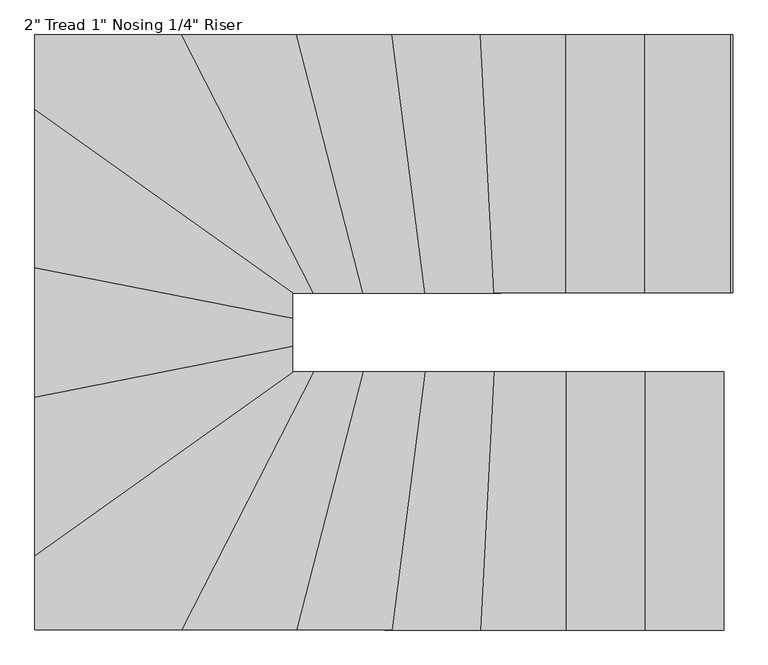
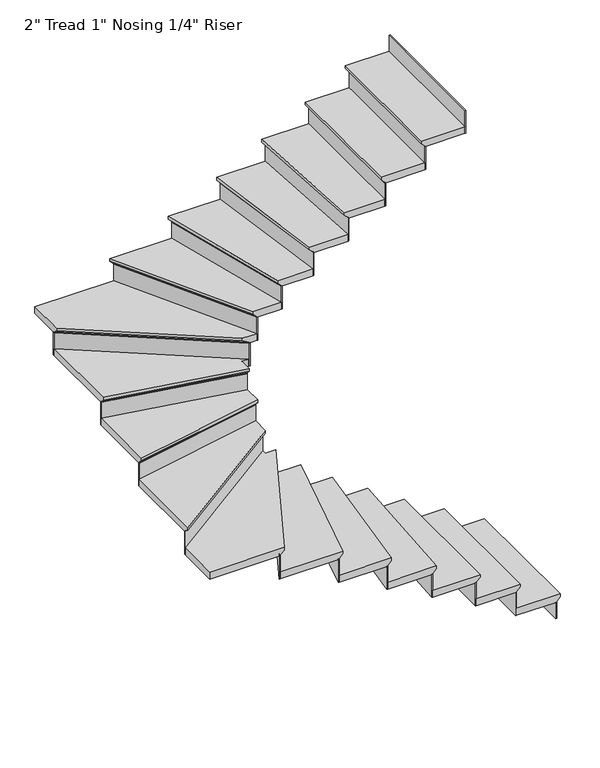
"""IFC4 building model written with IfcOpenShell, lengths in millimetres: stair flight geometry."""

from ifc_helpers import new_model, si_unit, origin, place, context, project, spatial, faceted_brep, source, transform, mapped, element, save


def stair_flight_428a4bf9(model_context):
    return source(origin(), model_context, "Body", "Brep", [
        faceted_brep([(-1761.7449167, -345.7070853, 6551.0833333), (-1761.7449167, -345.7070853, 6570.1333333), (-1761.7449167, -1260.1070853, 6570.1333333), (-1761.7449167, -1260.1070853, 6551.0833333), (-1787.1449167, -345.7070853, 6525.6833333), (-1787.1449167, -1260.1070853, 6525.6833333), (-2066.5449167, -345.7070853, 6570.1333333), (-2066.5449167, -1260.1070853, 6570.1333333), (-1787.1449167, -1260.1070853, 6519.3333333), (-2066.5449167, -1260.1070853, 6519.3333333), (-2066.5449167, -345.7070853, 6519.3333333), (-1787.1449167, -345.7070853, 6519.3333333)], [[[0, 1, 2, 3]], [[4, 0, 3, 5]], [[2, 1, 6, 7]], [[8, 9, 10, 11]], [[2, 7, 9, 8, 5, 3]], [[8, 11, 4, 5]], [[6, 1, 0, 4, 11, 10]], [[7, 6, 10, 9]]]),
        faceted_brep([(-1787.1449167, -345.7070853, 6519.3333333), (-1787.1449167, -345.7070853, 6400.8), (-1793.4949167, -345.7070853, 6400.8), (-1793.4949167, -345.7070853, 6519.3333333), (-1787.1449167, -1260.1070853, 6519.3333333), (-1793.4949167, -1260.1070853, 6519.3333333), (-1793.4949167, -1260.1070853, 6400.8), (-1787.1449167, -1260.1070853, 6400.8)], [[[0, 1, 2, 3]], [[4, 5, 6, 7]], [[1, 0, 4, 7]], [[2, 1, 7, 6]], [[3, 2, 6, 5]], [[0, 3, 5, 4]]]),
        faceted_brep([(-2066.5449167, -345.7070853, 6688.6666667), (-2066.5449167, -345.7070853, 6519.3333333), (-2072.8949167, -345.7070853, 6519.3333333), (-2072.8949167, -345.7070853, 6688.6666667), (-2066.5449167, -1260.1070853, 6688.6666667), (-2072.8949167, -1260.1070853, 6688.6666667), (-2072.8949167, -1260.1070853, 6519.3333333), (-2066.5449167, -1260.1070853, 6519.3333333)], [[[0, 1, 2, 3]], [[4, 5, 6, 7]], [[1, 0, 4, 7]], [[2, 1, 7, 6]], [[3, 2, 6, 5]], [[0, 3, 5, 4]]]),
        faceted_brep([(-2041.1449167, -1260.1070853, 6739.4666667), (-2041.1449167, -345.7070853, 6739.4666667), (-2345.9449167, -345.7070853, 6739.4666667), (-2345.9449167, -1260.1070853, 6739.4666667), (-2066.5449167, -1260.1070853, 6688.6666667), (-2345.9449167, -1260.1070853, 6688.6666667), (-2345.9449167, -345.7070853, 6688.6666667), (-2066.5449167, -345.7070853, 6688.6666667), (-2066.5449167, -1260.1070853, 6695.0166667), (-2041.1449167, -1260.1070853, 6720.4166667), (-2066.5449167, -345.7070853, 6695.0166667), (-2041.1449167, -345.7070853, 6720.4166667)], [[[0, 1, 2, 3]], [[4, 5, 6, 7]], [[0, 3, 5, 4, 8, 9]], [[4, 7, 10, 8]], [[2, 1, 11, 10, 7, 6]], [[3, 2, 6, 5]], [[11, 1, 0, 9]], [[10, 11, 9, 8]]]),
        faceted_brep([(-2345.9449167, -345.7070853, 6858.0), (-2345.9449167, -345.7070853, 6688.6666667), (-2352.2949167, -345.7070853, 6688.6666667), (-2352.2949167, -345.7070853, 6858.0), (-2345.9449167, -1260.1070853, 6858.0), (-2352.2949167, -1260.1070853, 6858.0), (-2352.2949167, -1260.1070853, 6688.6666667), (-2345.9449167, -1260.1070853, 6688.6666667)], [[[0, 1, 2, 3]], [[4, 5, 6, 7]], [[1, 0, 4, 7]], [[2, 1, 7, 6]], [[3, 2, 6, 5]], [[0, 3, 5, 4]]]),
        faceted_brep([(-2320.5449167, -1260.1070853, 6908.8), (-2320.5449167, -345.7070853, 6908.8), (-2601.6120781, -345.7070853, 6908.8), (-2649.1463485, -1260.1070853, 6908.8), (-2345.9449167, -1260.1070853, 6858.0), (-2649.1463485, -1260.1070853, 6858.0), (-2601.6120781, -345.7070853, 6858.0), (-2345.9449167, -345.7070853, 6858.0), (-2345.9449167, -1260.1070853, 6864.35), (-2320.5449167, -1260.1070853, 6889.75), (-2345.9449167, -345.7070853, 6864.35), (-2320.5449167, -345.7070853, 6889.75)], [[[0, 1, 2, 3]], [[4, 5, 6, 7]], [[0, 3, 5, 4, 8, 9]], [[4, 7, 10, 8]], [[2, 1, 11, 10, 7, 6]], [[3, 2, 6, 5]], [[11, 1, 0, 9]], [[10, 11, 9, 8]]]),
        faceted_brep([(-2601.6120781, -345.7070853, 7027.3333333), (-2601.6120781, -345.7070853, 6858.0), (-2607.9706523, -345.7070853, 6858.0), (-2607.9706523, -345.7070853, 7027.3333333), (-2649.1463485, -1260.1070853, 7027.3333333), (-2655.5049227, -1260.1070853, 7027.3333333), (-2655.5049227, -1260.1070853, 6858.0), (-2649.1463485, -1260.1070853, 6858.0)], [[[0, 1, 2, 3]], [[4, 5, 6, 7]], [[1, 0, 4, 7]], [[2, 1, 7, 6]], [[3, 2, 6, 5]], [[0, 3, 5, 4]]]),
        faceted_brep([(-2623.7120519, -1260.1070853, 7078.1333333), (-2576.1777815, -345.7070853, 7078.1333333), (-2845.778778, -345.7070853, 7078.1333333), (-2964.1348296, -1260.1070853, 7078.1333333), (-2649.1463485, -1260.1070853, 7027.3333333), (-2964.1348296, -1260.1070853, 7027.3333333), (-2845.778778, -345.7070853, 7027.3333333), (-2601.6120781, -345.7070853, 7027.3333333), (-2649.1463485, -1260.1070853, 7033.6833333), (-2623.7120519, -1260.1070853, 7059.0833333), (-2601.6120781, -345.7070853, 7033.6833333), (-2576.1777815, -345.7070853, 7059.0833333)], [[[0, 1, 2, 3]], [[4, 5, 6, 7]], [[0, 3, 5, 4, 8, 9]], [[4, 7, 10, 8]], [[2, 1, 11, 10, 7, 6]], [[3, 2, 6, 5]], [[11, 1, 0, 9]], [[10, 11, 9, 8]]]),
        faceted_brep([(-2845.778778, -345.7070853, 7196.6666667), (-2845.778778, -345.7070853, 7027.3333333), (-2852.1817497, -345.7070853, 7027.3333333), (-2852.1817497, -345.7070853, 7196.6666667), (-2964.1348296, -1260.1070853, 7196.6666667), (-2970.5378014, -1260.1070853, 7196.6666667), (-2970.5378014, -1260.1070853, 7027.3333333), (-2964.1348296, -1260.1070853, 7027.3333333)], [[[0, 1, 2, 3]], [[4, 5, 6, 7]], [[1, 0, 4, 7]], [[2, 1, 7, 6]], [[3, 2, 6, 5]], [[0, 3, 5, 4]]]),
        faceted_brep([(-2938.5229425, -1260.1070853, 7247.4666667), (-2820.1668908, -345.7070853, 7247.4666667), (-3067.4060004, -345.7070853, 7247.4666667), (-3302.5364478, -1260.1070853, 7247.4666667), (-2964.1348296, -1260.1070853, 7196.6666667), (-3302.5364478, -1260.1070853, 7196.6666667), (-3067.4060004, -345.7070853, 7196.6666667), (-2845.778778, -345.7070853, 7196.6666667), (-2964.1348296, -1260.1070853, 7203.0166667), (-2938.5229425, -1260.1070853, 7228.4166667), (-2845.778778, -345.7070853, 7203.0166667), (-2820.1668908, -345.7070853, 7228.4166667)], [[[0, 1, 2, 3]], [[4, 5, 6, 7]], [[0, 3, 5, 4, 8, 9]], [[4, 7, 10, 8]], [[2, 1, 11, 10, 7, 6]], [[3, 2, 6, 5]], [[11, 1, 0, 9]], [[10, 11, 9, 8]]]),
        faceted_brep([(-3067.4060004, -345.7070853, 7366.0), (-3067.4060004, -345.7070853, 7196.6666667), (-3073.9625773, -345.7070853, 7196.6666667), (-3073.9625773, -345.7070853, 7366.0), (-3302.5364478, -1260.1070853, 7366.0), (-3309.0930247, -1260.1070853, 7366.0), (-3309.0930247, -1260.1070853, 7196.6666667), (-3302.5364478, -1260.1070853, 7196.6666667)], [[[0, 1, 2, 3]], [[4, 5, 6, 7]], [[1, 0, 4, 7]], [[2, 1, 7, 6]], [[3, 2, 6, 5]], [[0, 3, 5, 4]]]),
        faceted_brep([(-3276.3101404, -1260.1070853, 7416.8), (-3041.179693, -345.7070853, 7416.8), (-3243.7526365, -345.7070853, 7416.8), (-3712.5772578, -1260.1070853, 7416.8), (-3302.5364478, -1260.1070853, 7366.0), (-3712.5772578, -1260.1070853, 7366.0), (-3243.7526365, -345.7070853, 7366.0), (-3067.4060004, -345.7070853, 7366.0), (-3302.5364478, -1260.1070853, 7372.35), (-3276.3101404, -1260.1070853, 7397.75), (-3067.4060004, -345.7070853, 7372.35), (-3041.179693, -345.7070853, 7397.75)], [[[0, 1, 2, 3]], [[4, 5, 6, 7]], [[0, 3, 5, 4, 8, 9]], [[4, 7, 10, 8]], [[2, 1, 11, 10, 7, 6]], [[3, 2, 6, 5]], [[11, 1, 0, 9]], [[10, 11, 9, 8]]]),
        faceted_brep([(-3243.7526365, -345.7070853, 7535.3333333), (-3243.7526365, -345.7070853, 7366.0), (-3250.8886197, -345.7070853, 7366.0), (-3250.8886197, -345.7070853, 7535.3333333), (-3712.5772578, -1260.1070853, 7535.3333333), (-3719.713241, -1260.1070853, 7535.3333333), (-3719.713241, -1260.1070853, 7366.0), (-3712.5772578, -1260.1070853, 7366.0)], [[[0, 1, 2, 3]], [[4, 5, 6, 7]], [[1, 0, 4, 7]], [[2, 1, 7, 6]], [[3, 2, 6, 5]], [[0, 3, 5, 4]]]),
        faceted_brep([(-4203.8766085, -966.4259516, 7586.1333333), (-4203.8766085, -1260.1070853, 7586.1333333), (-3684.0333253, -1260.1070853, 7586.1333333), (-3215.208704, -345.7070853, 7586.1333333), (-3289.4766085, -345.7070853, 7586.1333333), (-3289.4766085, -316.1520025, 7586.1333333), (-4203.8766085, -1260.1070853, 7535.3333333), (-4203.8766085, -966.4259516, 7535.3333333), (-3289.4766085, -316.1520025, 7535.3333333), (-3289.4766085, -345.7070853, 7535.3333333), (-3243.7526365, -345.7070853, 7535.3333333), (-3712.5772578, -1260.1070853, 7535.3333333), (-3712.5772578, -1260.1070853, 7541.6833333), (-3684.0333253, -1260.1070853, 7567.0833333), (-3243.7526365, -345.7070853, 7541.6833333), (-3215.208704, -345.7070853, 7567.0833333)], [[[0, 1, 2, 3, 4, 5]], [[6, 7, 8, 9, 10, 11]], [[1, 0, 7, 6]], [[2, 1, 6, 11, 12, 13]], [[11, 10, 14, 12]], [[4, 3, 15, 14, 10, 9]], [[5, 4, 9, 8]], [[0, 5, 8, 7]], [[15, 3, 2, 13]], [[14, 15, 13, 12]]]),
        faceted_brep([(-3289.4766085, -316.1520025, 7704.6666667), (-3289.4766085, -316.1520025, 7535.3333333), (-3289.4766085, -308.3600277, 7535.3333333), (-3289.4766085, -308.3600277, 7704.6666667), (-4203.8766085, -966.4259516, 7704.6666667), (-4203.8766085, -958.6339768, 7704.6666667), (-4203.8766085, -958.6339768, 7535.3333333), (-4203.8766085, -966.4259516, 7535.3333333)], [[[0, 1, 2, 3]], [[4, 5, 6, 7]], [[1, 0, 4, 7]], [[2, 1, 7, 6]], [[3, 2, 6, 5]], [[0, 3, 5, 4]]]),
        faceted_brep([(-4203.8766085, -997.5938508, 7755.4666667), (-3289.4766085, -347.3199017, 7755.4666667), (-3289.4766085, -229.6979154, 7755.4666667), (-4203.8766085, -409.9387717, 7755.4666667), (-4203.8766085, -966.4259516, 7704.6666667), (-4203.8766085, -409.9387717, 7704.6666667), (-3289.4766085, -229.6979154, 7704.6666667), (-3289.4766085, -316.1520025, 7704.6666667), (-4203.8766085, -966.4259516, 7711.0166667), (-4203.8766085, -997.5938508, 7736.4166667), (-3289.4766085, -316.1520025, 7711.0166667), (-3289.4766085, -347.3199017, 7736.4166667)], [[[0, 1, 2, 3]], [[4, 5, 6, 7]], [[0, 3, 5, 4, 8, 9]], [[4, 7, 10, 8]], [[2, 1, 11, 10, 7, 6]], [[3, 2, 6, 5]], [[11, 1, 0, 9]], [[10, 11, 9, 8]]]),
        faceted_brep([(-3289.4766085, -229.6979154, 7874.0), (-3289.4766085, -229.6979154, 7704.6666667), (-3289.4766085, -223.22573, 7704.6666667), (-3289.4766085, -223.22573, 7874.0), (-4203.8766085, -409.9387717, 7874.0), (-4203.8766085, -403.4665863, 7874.0), (-4203.8766085, -403.4665863, 7704.6666667), (-4203.8766085, -409.9387717, 7704.6666667)], [[[0, 1, 2, 3]], [[4, 5, 6, 7]], [[1, 0, 4, 7]], [[2, 1, 7, 6]], [[3, 2, 6, 5]], [[0, 3, 5, 4]]]),
        faceted_brep([(-4203.8766085, -435.8275135, 7924.8), (-3289.4766085, -255.5866572, 7924.8), (-3289.4766085, -130.5387717, 7924.8), (-4203.8766085, 49.7020846, 7924.8), (-4203.8766085, -409.9387717, 7874.0), (-4203.8766085, 49.7020846, 7874.0), (-3289.4766085, -130.5387717, 7874.0), (-3289.4766085, -229.6979154, 7874.0), (-4203.8766085, -409.9387717, 7880.35), (-4203.8766085, -435.8275135, 7905.75), (-3289.4766085, -229.6979154, 7880.35), (-3289.4766085, -255.5866572, 7905.75)], [[[0, 1, 2, 3]], [[4, 5, 6, 7]], [[0, 3, 5, 4, 8, 9]], [[4, 7, 10, 8]], [[2, 1, 11, 10, 7, 6]], [[3, 2, 6, 5]], [[11, 1, 0, 9]], [[10, 11, 9, 8]]]),
        faceted_brep([(-3289.4766085, -130.5387717, 8043.3333333), (-3289.4766085, -130.5387717, 7874.0), (-3289.4766085, -124.0665863, 7874.0), (-3289.4766085, -124.0665863, 8043.3333333), (-4203.8766085, 49.7020846, 8043.3333333), (-4203.8766085, 56.17427, 8043.3333333), (-4203.8766085, 56.17427, 7874.0), (-4203.8766085, 49.7020846, 7874.0)], [[[0, 1, 2, 3]], [[4, 5, 6, 7]], [[1, 0, 4, 7]], [[2, 1, 7, 6]], [[3, 2, 6, 5]], [[0, 3, 5, 4]]]),
        faceted_brep([(-4203.8766085, 23.8133428, 8094.1333333), (-3289.4766085, -156.4275135, 8094.1333333), (-3289.4766085, -66.3070853, 8094.1333333), (-3243.381134, -66.3070853, 8094.1333333), (-4203.8766085, 616.7475793, 8094.1333333), (-4203.8766085, 49.7020846, 8043.3333333), (-4203.8766085, 616.7475793, 8043.3333333), (-3243.381134, -66.3070853, 8043.3333333), (-3289.4766085, -66.3070853, 8043.3333333), (-3289.4766085, -130.5387717, 8043.3333333), (-4203.8766085, 49.7020846, 8049.6833333), (-4203.8766085, 23.8133428, 8075.0833333), (-3289.4766085, -130.5387717, 8049.6833333), (-3289.4766085, -156.4275135, 8075.0833333)], [[[0, 1, 2, 3, 4]], [[5, 6, 7, 8, 9]], [[0, 4, 6, 5, 10, 11]], [[5, 9, 12, 10]], [[2, 1, 13, 12, 9, 8]], [[3, 2, 8, 7]], [[4, 3, 7, 6]], [[13, 1, 0, 11]], [[12, 13, 11, 10]]]),
        faceted_brep([(-3243.381134, -66.3070853, 8212.6666667), (-3243.381134, -66.3070853, 8043.3333333), (-3232.4242415, -66.3070853, 8043.3333333), (-3232.4242415, -66.3070853, 8212.6666667), (-4203.8766085, 616.7475793, 8212.6666667), (-4203.8766085, 624.5395541, 8212.6666667), (-4203.8766085, 624.5395541, 8043.3333333), (-4203.8766085, 616.7475793, 8043.3333333)], [[[0, 1, 2, 3]], [[4, 5, 6, 7]], [[1, 0, 4, 7]], [[2, 1, 7, 6]], [[3, 2, 6, 5]], [[0, 3, 5, 4]]]),
        faceted_brep([(-3655.4893928, 848.0929147, 8263.4666667), (-4203.8766085, 848.0929147, 8263.4666667), (-4203.8766085, 585.5796802, 8263.4666667), (-3287.208704, -66.3070853, 8263.4666667), (-3186.6647715, -66.3070853, 8263.4666667), (-4203.8766085, 848.0929147, 8212.6666667), (-3655.4893928, 848.0929147, 8212.6666667), (-3186.6647715, -66.3070853, 8212.6666667), (-3243.381134, -66.3070853, 8212.6666667), (-4203.8766085, 616.7475793, 8212.6666667), (-4203.8766085, 616.7475793, 8219.0166667), (-4203.8766085, 585.5796802, 8244.4166667), (-3243.381134, -66.3070853, 8219.0166667), (-3287.208704, -66.3070853, 8244.4166667)], [[[0, 1, 2, 3, 4]], [[5, 6, 7, 8, 9]], [[1, 0, 6, 5]], [[2, 1, 5, 9, 10, 11]], [[9, 8, 12, 10]], [[4, 3, 13, 12, 8, 7]], [[0, 4, 7, 6]], [[13, 3, 2, 11]], [[12, 13, 11, 10]]]),
        faceted_brep([(-3186.6647715, -66.3070853, 8382.0), (-3186.6647715, -66.3070853, 8212.6666667), (-3179.5287883, -66.3070853, 8212.6666667), (-3179.5287883, -66.3070853, 8382.0), (-3655.4893928, 848.0929147, 8382.0), (-3648.3534096, 848.0929147, 8382.0), (-3648.3534096, 848.0929147, 8212.6666667), (-3655.4893928, 848.0929147, 8212.6666667)], [[[0, 1, 2, 3]], [[4, 5, 6, 7]], [[1, 0, 4, 7]], [[2, 1, 7, 6]], [[3, 2, 6, 5]], [[0, 3, 5, 4]]]),
        faceted_brep([(-3684.0333253, 848.0929147, 8432.8), (-3215.208704, -66.3070853, 8432.8), (-3014.9533855, -66.3070853, 8432.8), (-3250.0838329, 848.0929147, 8432.8), (-3655.4893928, 848.0929147, 8382.0), (-3250.0838329, 848.0929147, 8382.0), (-3014.9533855, -66.3070853, 8382.0), (-3186.6647715, -66.3070853, 8382.0), (-3655.4893928, 848.0929147, 8388.35), (-3684.0333253, 848.0929147, 8413.75), (-3186.6647715, -66.3070853, 8388.35), (-3215.208704, -66.3070853, 8413.75)], [[[0, 1, 2, 3]], [[4, 5, 6, 7]], [[0, 3, 5, 4, 8, 9]], [[4, 7, 10, 8]], [[2, 1, 11, 10, 7, 6]], [[3, 2, 6, 5]], [[11, 1, 0, 9]], [[10, 11, 9, 8]]]),
        faceted_brep([(-3014.9533855, -66.3070853, 8551.3333333), (-3014.9533855, -66.3070853, 8382.0), (-3008.3968086, -66.3070853, 8382.0), (-3008.3968086, -66.3070853, 8551.3333333), (-3250.0838329, 848.0929147, 8551.3333333), (-3243.5272561, 848.0929147, 8551.3333333), (-3243.5272561, 848.0929147, 8382.0), (-3250.0838329, 848.0929147, 8382.0)], [[[0, 1, 2, 3]], [[4, 5, 6, 7]], [[1, 0, 4, 7]], [[2, 1, 7, 6]], [[3, 2, 6, 5]], [[0, 3, 5, 4]]]),
        faceted_brep([(-3276.3101404, 848.0929147, 8602.1333333), (-3041.179693, -66.3070853, 8602.1333333), (-2794.5550037, -66.3070853, 8602.1333333), (-2912.9110554, 848.0929147, 8602.1333333), (-3250.0838329, 848.0929147, 8551.3333333), (-2912.9110554, 848.0929147, 8551.3333333), (-2794.5550037, -66.3070853, 8551.3333333), (-3014.9533855, -66.3070853, 8551.3333333), (-3250.0838329, 848.0929147, 8557.6833333), (-3276.3101404, 848.0929147, 8583.0833333), (-3014.9533855, -66.3070853, 8557.6833333), (-3041.179693, -66.3070853, 8583.0833333)], [[[0, 1, 2, 3]], [[4, 5, 6, 7]], [[0, 3, 5, 4, 8, 9]], [[4, 7, 10, 8]], [[2, 1, 11, 10, 7, 6]], [[3, 2, 6, 5]], [[11, 1, 0, 9]], [[10, 11, 9, 8]]]),
        faceted_brep([(-2794.5550037, -66.3070853, 8720.6666667), (-2794.5550037, -66.3070853, 8551.3333333), (-2788.152032, -66.3070853, 8551.3333333), (-2788.152032, -66.3070853, 8720.6666667), (-2912.9110554, 848.0929147, 8720.6666667), (-2906.5080836, 848.0929147, 8720.6666667), (-2906.5080836, 848.0929147, 8551.3333333), (-2912.9110554, 848.0929147, 8551.3333333)], [[[0, 1, 2, 3]], [[4, 5, 6, 7]], [[1, 0, 4, 7]], [[2, 1, 7, 6]], [[3, 2, 6, 5]], [[0, 3, 5, 4]]]),
        faceted_brep([(-2938.5229425, 848.0929147, 8771.4666667), (-2820.1668908, -66.3070853, 8771.4666667), (-2550.7434848, -66.3070853, 8771.4666667), (-2598.2777552, 848.0929147, 8771.4666667), (-2912.9110554, 848.0929147, 8720.6666667), (-2598.2777552, 848.0929147, 8720.6666667), (-2550.7434848, -66.3070853, 8720.6666667), (-2794.5550037, -66.3070853, 8720.6666667), (-2912.9110554, 848.0929147, 8727.0166667), (-2938.5229425, 848.0929147, 8752.4166667), (-2794.5550037, -66.3070853, 8727.0166667), (-2820.1668908, -66.3070853, 8752.4166667)], [[[0, 1, 2, 3]], [[4, 5, 6, 7]], [[0, 3, 5, 4, 8, 9]], [[4, 7, 10, 8]], [[2, 1, 11, 10, 7, 6]], [[3, 2, 6, 5]], [[11, 1, 0, 9]], [[10, 11, 9, 8]]]),
        faceted_brep([(-2550.7434848, -66.3070853, 8890.0), (-2550.7434848, -66.3070853, 8720.6666667), (-2544.3849106, -66.3070853, 8720.6666667), (-2544.3849106, -66.3070853, 8890.0), (-2598.2777552, 848.0929147, 8890.0), (-2591.9191811, 848.0929147, 8890.0), (-2591.9191811, 848.0929147, 8720.6666667), (-2598.2777552, 848.0929147, 8720.6666667)], [[[0, 1, 2, 3]], [[4, 5, 6, 7]], [[1, 0, 4, 7]], [[2, 1, 7, 6]], [[3, 2, 6, 5]], [[0, 3, 5, 4]]]),
        faceted_brep([(-2623.7120519, 848.0929147, 8940.8), (-2576.1777815, -66.3070853, 8940.8), (-2295.1449167, -66.3070853, 8940.8), (-2295.1449167, 848.0929147, 8940.8), (-2598.2777552, 848.0929147, 8890.0), (-2295.1449167, 848.0929147, 8890.0), (-2295.1449167, -66.3070853, 8890.0), (-2550.7434848, -66.3070853, 8890.0), (-2598.2777552, 848.0929147, 8896.35), (-2623.7120519, 848.0929147, 8921.75), (-2550.7434848, -66.3070853, 8896.35), (-2576.1777815, -66.3070853, 8921.75)], [[[0, 1, 2, 3]], [[4, 5, 6, 7]], [[0, 3, 5, 4, 8, 9]], [[4, 7, 10, 8]], [[2, 1, 11, 10, 7, 6]], [[3, 2, 6, 5]], [[11, 1, 0, 9]], [[10, 11, 9, 8]]]),
        faceted_brep([(-2295.1449167, -66.3070853, 9059.3333333), (-2295.1449167, -66.3070853, 8890.0), (-2288.7949167, -66.3070853, 8890.0), (-2288.7949167, -66.3070853, 9059.3333333), (-2295.1449167, 848.0929147, 9059.3333333), (-2288.7949167, 848.0929147, 9059.3333333), (-2288.7949167, 848.0929147, 8890.0), (-2295.1449167, 848.0929147, 8890.0)], [[[0, 1, 2, 3]], [[4, 5, 6, 7]], [[1, 0, 4, 7]], [[2, 1, 7, 6]], [[3, 2, 6, 5]], [[0, 3, 5, 4]]]),
        faceted_brep([(-2320.5449167, 848.0929147, 9110.1333333), (-2320.5449167, -66.3070853, 9110.1333333), (-2015.7449167, -66.3070853, 9110.1333333), (-2015.7449167, 848.0929147, 9110.1333333), (-2295.1449167, 848.0929147, 9059.3333333), (-2015.7449167, 848.0929147, 9059.3333333), (-2015.7449167, -66.3070853, 9059.3333333), (-2295.1449167, -66.3070853, 9059.3333333), (-2295.1449167, 848.0929147, 9065.6833333), (-2320.5449167, 848.0929147, 9091.0833333), (-2295.1449167, -66.3070853, 9065.6833333), (-2320.5449167, -66.3070853, 9091.0833333)], [[[0, 1, 2, 3]], [[4, 5, 6, 7]], [[0, 3, 5, 4, 8, 9]], [[4, 7, 10, 8]], [[2, 1, 11, 10, 7, 6]], [[3, 2, 6, 5]], [[11, 1, 0, 9]], [[10, 11, 9, 8]]]),
        faceted_brep([(-2015.7449167, -66.3070853, 9228.6666667), (-2015.7449167, -66.3070853, 9059.3333333), (-2009.3949167, -66.3070853, 9059.3333333), (-2009.3949167, -66.3070853, 9228.6666667), (-2015.7449167, 848.0929147, 9228.6666667), (-2009.3949167, 848.0929147, 9228.6666667), (-2009.3949167, 848.0929147, 9059.3333333), (-2015.7449167, 848.0929147, 9059.3333333)], [[[0, 1, 2, 3]], [[4, 5, 6, 7]], [[1, 0, 4, 7]], [[2, 1, 7, 6]], [[3, 2, 6, 5]], [[0, 3, 5, 4]]]),
        faceted_brep([(-1736.3449167, -66.3070853, 9398.0), (-1736.3449167, -66.3070853, 9228.6666667), (-1729.9949167, -66.3070853, 9228.6666667), (-1729.9949167, -66.3070853, 9398.0), (-1736.3449167, 848.0929147, 9398.0), (-1729.9949167, 848.0929147, 9398.0), (-1729.9949167, 848.0929147, 9228.6666667), (-1736.3449167, 848.0929147, 9228.6666667)], [[[0, 1, 2, 3]], [[4, 5, 6, 7]], [[1, 0, 4, 7]], [[2, 1, 7, 6]], [[3, 2, 6, 5]], [[0, 3, 5, 4]]]),
        faceted_brep([(-2041.1449167, 848.0929147, 9279.4666667), (-2041.1449167, -66.3070853, 9279.4666667), (-1736.3449167, -66.3070853, 9279.4666667), (-1736.3449167, 848.0929147, 9279.4666667), (-2015.7449167, 848.0929147, 9228.6666667), (-1736.3449167, 848.0929147, 9228.6666667), (-1736.3449167, -66.3070853, 9228.6666667), (-2015.7449167, -66.3070853, 9228.6666667), (-2015.7449167, 848.0929147, 9235.0166667), (-2041.1449167, 848.0929147, 9260.4166667), (-2015.7449167, -66.3070853, 9235.0166667), (-2041.1449167, -66.3070853, 9260.4166667)], [[[0, 1, 2, 3]], [[4, 5, 6, 7]], [[0, 3, 5, 4, 8, 9]], [[4, 7, 10, 8]], [[2, 1, 11, 10, 7, 6]], [[3, 2, 6, 5]], [[11, 1, 0, 9]], [[10, 11, 9, 8]]]),
    ])


if __name__ == "__main__":
    model = new_model("IFC4")
    model_context = context("Model", 3, world=origin())
    ifc_project = project(units=[si_unit("LENGTHUNIT", "METRE", prefix="MILLI")], contexts=[model_context])
    site = spatial("IfcSite", under=ifc_project)
    building = spatial("IfcBuilding", under=site)
    placement = place(None, origin())
    stair_flight_shape = stair_flight_428a4bf9(model_context)
    element("IfcStairFlight", 1, ObjectType="2\" Tread 1\" Nosing 1/4\" Riser", at=placement, inside=building, context=model_context, shape_type="MappedRepresentation", body=[
        mapped(stair_flight_shape, transform((0.0, 0.0, 0.0), x_axis=(1.0, 0.0, 0.0), y_axis=(0.0, 1.0, 0.0), z_axis=(0.0, 0.0, 1.0))),
    ])
    save(model, "model.ifc")
